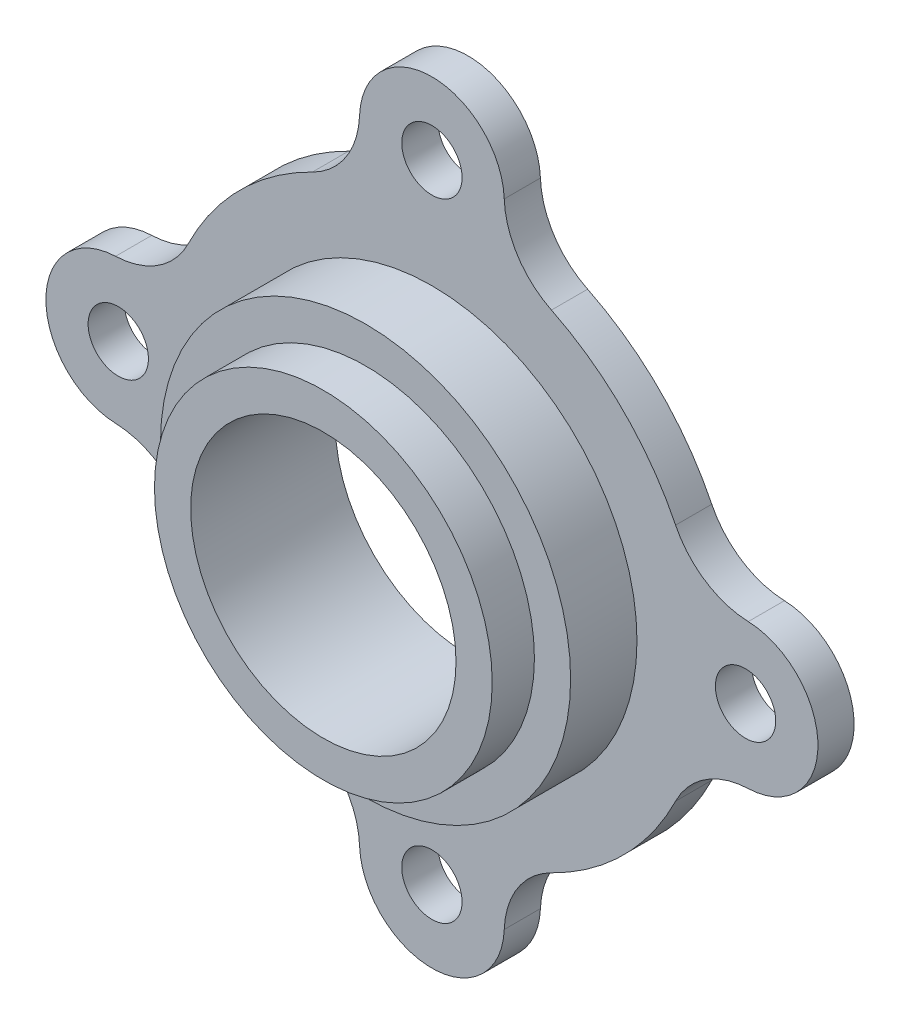
ISO-10303-21;
HEADER;
FILE_DESCRIPTION(('STEP AP214'),'2;1');
FILE_NAME('part.step','',(''),(''),'','','');
FILE_SCHEMA(('AUTOMOTIVE_DESIGN { 1 0 10303 214 1 1 1 1 }'));
ENDSEC;
DATA;
#1=APPLICATION_CONTEXT('core data for automotive mechanical design processes');
#2=APPLICATION_PROTOCOL_DEFINITION('international standard','automotive_design',2000,#1);
#3=PRODUCT_CONTEXT('',#1,'mechanical');
#4=PRODUCT('Part','Part','',(#3));
#5=PRODUCT_RELATED_PRODUCT_CATEGORY('part','',(#4));
#6=PRODUCT_DEFINITION_FORMATION('','',#4);
#7=PRODUCT_DEFINITION_CONTEXT('part definition',#1,'design');
#8=PRODUCT_DEFINITION('design','',#6,#7);
#9=PRODUCT_DEFINITION_SHAPE('','',#8);
#10=(LENGTH_UNIT() NAMED_UNIT(*) SI_UNIT(.MILLI.,.METRE.));
#11=(NAMED_UNIT(*) PLANE_ANGLE_UNIT() SI_UNIT($,.RADIAN.));
#12=(NAMED_UNIT(*) SI_UNIT($,.STERADIAN.) SOLID_ANGLE_UNIT());
#13=UNCERTAINTY_MEASURE_WITH_UNIT(LENGTH_MEASURE(1.E-05),#10,'distance_accuracy_value','');
#14=(GEOMETRIC_REPRESENTATION_CONTEXT(3) GLOBAL_UNCERTAINTY_ASSIGNED_CONTEXT((#13)) GLOBAL_UNIT_ASSIGNED_CONTEXT((#10,
#11,#12)) REPRESENTATION_CONTEXT('',''));
#15=CARTESIAN_POINT('',(0.,0.,0.));
#16=DIRECTION('',(0.,0.,1.));
#17=DIRECTION('',(1.,0.,0.));
#18=AXIS2_PLACEMENT_3D('',#15,#16,#17);
#19=CARTESIAN_POINT('',(12.9909281828426,26.4855769230769,3.));
#20=DIRECTION('',(0.,0.,-1.));
#21=DIRECTION('',(-1.,0.,0.));
#22=AXIS2_PLACEMENT_3D('',#19,#20,#21);
#23=CYLINDRICAL_SURFACE('',#22,7.);
#24=CARTESIAN_POINT('',(12.9909281828426,26.4855769230769,0.));
#25=DIRECTION('',(0.,0.,-1.));
#26=DIRECTION('',(-1.,0.,0.));
#27=AXIS2_PLACEMENT_3D('',#24,#25,#26);
#28=CIRCLE('',#27,7.);
#29=CARTESIAN_POINT('',(9.90833505471048,20.2008637548892,0.));
#30=VERTEX_POINT('',#29);
#31=CARTESIAN_POINT('',(5.99581300746583,26.2241124260355,0.));
#32=VERTEX_POINT('',#31);
#33=EDGE_CURVE('E186',#30,#32,#28,.T.);
#34=ORIENTED_EDGE('',*,*,#33,.T.);
#35=DIRECTION('',(0.,0.,-1.));
#36=VECTOR('',#35,1.);
#37=CARTESIAN_POINT('',(5.99581300746583,26.2241124260355,3.));
#38=LINE('',#37,#36);
#39=CARTESIAN_POINT('',(5.99581300746583,26.2241124260355,3.));
#40=VERTEX_POINT('',#39);
#41=EDGE_CURVE('E256',#40,#32,#38,.T.);
#42=ORIENTED_EDGE('',*,*,#41,.F.);
#43=CARTESIAN_POINT('',(12.9909281828426,26.4855769230769,3.));
#44=DIRECTION('',(0.,0.,-1.));
#45=DIRECTION('',(-1.,0.,0.));
#46=AXIS2_PLACEMENT_3D('',#43,#44,#45);
#47=CIRCLE('',#46,7.);
#48=CARTESIAN_POINT('',(9.90833505471048,20.2008637548892,3.));
#49=VERTEX_POINT('',#48);
#50=EDGE_CURVE('E222',#49,#40,#47,.T.);
#51=ORIENTED_EDGE('',*,*,#50,.F.);
#52=DIRECTION('',(0.,0.,-1.));
#53=VECTOR('',#52,1.);
#54=CARTESIAN_POINT('',(9.90833505471048,20.2008637548892,3.));
#55=LINE('',#54,#53);
#56=EDGE_CURVE('E188',#49,#30,#55,.T.);
#57=ORIENTED_EDGE('',*,*,#56,.T.);
#58=EDGE_LOOP('',(#34,#42,#51,#57));
#59=FACE_BOUND('',#58,.T.);
#60=ADVANCED_FACE('F43',(#59),#23,.F.);
#61=CARTESIAN_POINT('',(0.,26.,3.));
#62=DIRECTION('',(0.,0.,-1.));
#63=DIRECTION('',(-1.,0.,0.));
#64=AXIS2_PLACEMENT_3D('',#61,#62,#63);
#65=CYLINDRICAL_SURFACE('',#64,5.99999999999999);
#66=CARTESIAN_POINT('',(0.,26.,0.));
#67=DIRECTION('',(0.,0.,1.));
#68=DIRECTION('',(1.,0.,0.));
#69=AXIS2_PLACEMENT_3D('',#66,#67,#68);
#70=CIRCLE('',#69,5.99999999999999);
#71=CARTESIAN_POINT('',(-5.99581300746583,26.2241124260355,0.));
#72=VERTEX_POINT('',#71);
#73=EDGE_CURVE('E193',#32,#72,#70,.T.);
#74=ORIENTED_EDGE('',*,*,#73,.T.);
#75=DIRECTION('',(0.,0.,-1.));
#76=VECTOR('',#75,1.);
#77=CARTESIAN_POINT('',(-5.99581300746583,26.2241124260355,3.));
#78=LINE('',#77,#76);
#79=CARTESIAN_POINT('',(-5.99581300746583,26.2241124260355,3.));
#80=VERTEX_POINT('',#79);
#81=EDGE_CURVE('E254',#80,#72,#78,.T.);
#82=ORIENTED_EDGE('',*,*,#81,.F.);
#83=CARTESIAN_POINT('',(0.,26.,3.));
#84=DIRECTION('',(0.,0.,1.));
#85=DIRECTION('',(1.,0.,0.));
#86=AXIS2_PLACEMENT_3D('',#83,#84,#85);
#87=CIRCLE('',#86,5.99999999999999);
#88=EDGE_CURVE('E129',#40,#80,#87,.T.);
#89=ORIENTED_EDGE('',*,*,#88,.F.);
#90=ORIENTED_EDGE('',*,*,#41,.T.);
#91=EDGE_LOOP('',(#74,#82,#89,#90));
#92=FACE_BOUND('',#91,.T.);
#93=ADVANCED_FACE('F345',(#92),#65,.T.);
#94=CARTESIAN_POINT('',(-12.9909281828426,26.4855769230769,3.));
#95=DIRECTION('',(0.,0.,-1.));
#96=DIRECTION('',(-1.,0.,0.));
#97=AXIS2_PLACEMENT_3D('',#94,#95,#96);
#98=CYLINDRICAL_SURFACE('',#97,7.);
#99=CARTESIAN_POINT('',(-12.9909281828426,26.4855769230769,0.));
#100=DIRECTION('',(0.,0.,-1.));
#101=DIRECTION('',(-1.,0.,0.));
#102=AXIS2_PLACEMENT_3D('',#99,#100,#101);
#103=CIRCLE('',#102,7.);
#104=CARTESIAN_POINT('',(-9.90833505471049,20.2008637548892,0.));
#105=VERTEX_POINT('',#104);
#106=EDGE_CURVE('E198',#72,#105,#103,.T.);
#107=ORIENTED_EDGE('',*,*,#106,.T.);
#108=DIRECTION('',(0.,0.,-1.));
#109=VECTOR('',#108,1.);
#110=CARTESIAN_POINT('',(-9.90833505471049,20.2008637548892,3.));
#111=LINE('',#110,#109);
#112=CARTESIAN_POINT('',(-9.90833505471049,20.2008637548892,3.));
#113=VERTEX_POINT('',#112);
#114=EDGE_CURVE('E252',#113,#105,#111,.T.);
#115=ORIENTED_EDGE('',*,*,#114,.F.);
#116=CARTESIAN_POINT('',(-12.9909281828426,26.4855769230769,3.));
#117=DIRECTION('',(0.,0.,-1.));
#118=DIRECTION('',(-1.,0.,0.));
#119=AXIS2_PLACEMENT_3D('',#116,#117,#118);
#120=CIRCLE('',#119,7.);
#121=EDGE_CURVE('E294',#80,#113,#120,.T.);
#122=ORIENTED_EDGE('',*,*,#121,.F.);
#123=ORIENTED_EDGE('',*,*,#81,.T.);
#124=EDGE_LOOP('',(#107,#115,#122,#123));
#125=FACE_BOUND('',#124,.T.);
#126=ADVANCED_FACE('F347',(#125),#98,.F.);
#127=CARTESIAN_POINT('',(0.,0.,3.));
#128=DIRECTION('',(0.,0.,-1.));
#129=DIRECTION('',(-1.,0.,0.));
#130=AXIS2_PLACEMENT_3D('',#127,#128,#129);
#131=CYLINDRICAL_SURFACE('',#130,22.5);
#132=CARTESIAN_POINT('',(0.,0.,0.));
#133=DIRECTION('',(0.,0.,1.));
#134=DIRECTION('',(1.,0.,0.));
#135=AXIS2_PLACEMENT_3D('',#132,#133,#134);
#136=CIRCLE('',#135,22.5);
#137=CARTESIAN_POINT('',(-20.2008637548892,9.90833505471048,0.));
#138=VERTEX_POINT('',#137);
#139=EDGE_CURVE('E196',#105,#138,#136,.T.);
#140=ORIENTED_EDGE('',*,*,#139,.T.);
#141=DIRECTION('',(0.,0.,-1.));
#142=VECTOR('',#141,1.);
#143=CARTESIAN_POINT('',(-20.2008637548892,9.90833505471048,3.));
#144=LINE('',#143,#142);
#145=CARTESIAN_POINT('',(-20.2008637548892,9.90833505471048,3.));
#146=VERTEX_POINT('',#145);
#147=EDGE_CURVE('E249',#146,#138,#144,.T.);
#148=ORIENTED_EDGE('',*,*,#147,.F.);
#149=CARTESIAN_POINT('',(0.,0.,3.));
#150=DIRECTION('',(0.,0.,1.));
#151=DIRECTION('',(1.,0.,0.));
#152=AXIS2_PLACEMENT_3D('',#149,#150,#151);
#153=CIRCLE('',#152,22.5);
#154=EDGE_CURVE('E298',#113,#146,#153,.T.);
#155=ORIENTED_EDGE('',*,*,#154,.F.);
#156=ORIENTED_EDGE('',*,*,#114,.T.);
#157=EDGE_LOOP('',(#140,#148,#155,#156));
#158=FACE_BOUND('',#157,.T.);
#159=ADVANCED_FACE('F348',(#158),#131,.T.);
#160=CARTESIAN_POINT('',(-26.4855769230769,12.9909281828426,3.));
#161=DIRECTION('',(0.,0.,-1.));
#162=DIRECTION('',(-1.,0.,0.));
#163=AXIS2_PLACEMENT_3D('',#160,#161,#162);
#164=CYLINDRICAL_SURFACE('',#163,7.);
#165=CARTESIAN_POINT('',(-26.4855769230769,12.9909281828426,0.));
#166=DIRECTION('',(0.,0.,-1.));
#167=DIRECTION('',(-1.,0.,0.));
#168=AXIS2_PLACEMENT_3D('',#165,#166,#167);
#169=CIRCLE('',#168,7.);
#170=CARTESIAN_POINT('',(-26.2241124260355,5.99581300746583,0.));
#171=VERTEX_POINT('',#170);
#172=EDGE_CURVE('E199',#138,#171,#169,.T.);
#173=ORIENTED_EDGE('',*,*,#172,.T.);
#174=DIRECTION('',(0.,0.,-1.));
#175=VECTOR('',#174,1.);
#176=CARTESIAN_POINT('',(-26.2241124260355,5.99581300746583,3.));
#177=LINE('',#176,#175);
#178=CARTESIAN_POINT('',(-26.2241124260355,5.99581300746583,3.));
#179=VERTEX_POINT('',#178);
#180=EDGE_CURVE('E247',#179,#171,#177,.T.);
#181=ORIENTED_EDGE('',*,*,#180,.F.);
#182=CARTESIAN_POINT('',(-26.4855769230769,12.9909281828426,3.));
#183=DIRECTION('',(0.,0.,-1.));
#184=DIRECTION('',(-1.,0.,0.));
#185=AXIS2_PLACEMENT_3D('',#182,#183,#184);
#186=CIRCLE('',#185,7.);
#187=EDGE_CURVE('E297',#146,#179,#186,.T.);
#188=ORIENTED_EDGE('',*,*,#187,.F.);
#189=ORIENTED_EDGE('',*,*,#147,.T.);
#190=EDGE_LOOP('',(#173,#181,#188,#189));
#191=FACE_BOUND('',#190,.T.);
#192=ADVANCED_FACE('F357',(#191),#164,.F.);
#193=CARTESIAN_POINT('',(-26.,0.,3.));
#194=DIRECTION('',(0.,0.,-1.));
#195=DIRECTION('',(-1.,0.,0.));
#196=AXIS2_PLACEMENT_3D('',#193,#194,#195);
#197=CYLINDRICAL_SURFACE('',#196,5.99999999999999);
#198=CARTESIAN_POINT('',(-26.,0.,0.));
#199=DIRECTION('',(0.,0.,1.));
#200=DIRECTION('',(1.,0.,0.));
#201=AXIS2_PLACEMENT_3D('',#198,#199,#200);
#202=CIRCLE('',#201,5.99999999999999);
#203=CARTESIAN_POINT('',(-26.2241124260355,-5.99581300746583,0.));
#204=VERTEX_POINT('',#203);
#205=EDGE_CURVE('E205',#171,#204,#202,.T.);
#206=ORIENTED_EDGE('',*,*,#205,.T.);
#207=DIRECTION('',(0.,0.,-1.));
#208=VECTOR('',#207,1.);
#209=CARTESIAN_POINT('',(-26.2241124260355,-5.99581300746583,3.));
#210=LINE('',#209,#208);
#211=CARTESIAN_POINT('',(-26.2241124260355,-5.99581300746583,3.));
#212=VERTEX_POINT('',#211);
#213=EDGE_CURVE('E242',#212,#204,#210,.T.);
#214=ORIENTED_EDGE('',*,*,#213,.F.);
#215=CARTESIAN_POINT('',(-26.,0.,3.));
#216=DIRECTION('',(0.,0.,1.));
#217=DIRECTION('',(1.,0.,0.));
#218=AXIS2_PLACEMENT_3D('',#215,#216,#217);
#219=CIRCLE('',#218,5.99999999999999);
#220=EDGE_CURVE('E296',#179,#212,#219,.T.);
#221=ORIENTED_EDGE('',*,*,#220,.F.);
#222=ORIENTED_EDGE('',*,*,#180,.T.);
#223=EDGE_LOOP('',(#206,#214,#221,#222));
#224=FACE_BOUND('',#223,.T.);
#225=ADVANCED_FACE('F356',(#224),#197,.T.);
#226=CARTESIAN_POINT('',(-26.4855769230769,-12.9909281828426,3.));
#227=DIRECTION('',(0.,0.,-1.));
#228=DIRECTION('',(-1.,0.,0.));
#229=AXIS2_PLACEMENT_3D('',#226,#227,#228);
#230=CYLINDRICAL_SURFACE('',#229,7.);
#231=CARTESIAN_POINT('',(-26.4855769230769,-12.9909281828426,0.));
#232=DIRECTION('',(0.,0.,-1.));
#233=DIRECTION('',(1.,0.,0.));
#234=AXIS2_PLACEMENT_3D('',#231,#232,#233);
#235=CIRCLE('',#234,7.);
#236=CARTESIAN_POINT('',(-20.2008637548892,-9.90833505471048,0.));
#237=VERTEX_POINT('',#236);
#238=EDGE_CURVE('E204',#204,#237,#235,.T.);
#239=ORIENTED_EDGE('',*,*,#238,.T.);
#240=DIRECTION('',(0.,0.,-1.));
#241=VECTOR('',#240,1.);
#242=CARTESIAN_POINT('',(-20.2008637548892,-9.90833505471048,3.));
#243=LINE('',#242,#241);
#244=CARTESIAN_POINT('',(-20.2008637548892,-9.90833505471048,3.));
#245=VERTEX_POINT('',#244);
#246=EDGE_CURVE('E238',#245,#237,#243,.T.);
#247=ORIENTED_EDGE('',*,*,#246,.F.);
#248=CARTESIAN_POINT('',(-26.4855769230769,-12.9909281828426,3.));
#249=DIRECTION('',(0.,0.,-1.));
#250=DIRECTION('',(1.,0.,0.));
#251=AXIS2_PLACEMENT_3D('',#248,#249,#250);
#252=CIRCLE('',#251,7.);
#253=EDGE_CURVE('E305',#212,#245,#252,.T.);
#254=ORIENTED_EDGE('',*,*,#253,.F.);
#255=ORIENTED_EDGE('',*,*,#213,.T.);
#256=EDGE_LOOP('',(#239,#247,#254,#255));
#257=FACE_BOUND('',#256,.T.);
#258=ADVANCED_FACE('F365',(#257),#230,.F.);
#259=CARTESIAN_POINT('',(0.,0.,3.));
#260=DIRECTION('',(0.,0.,-1.));
#261=DIRECTION('',(-1.,0.,0.));
#262=AXIS2_PLACEMENT_3D('',#259,#260,#261);
#263=CYLINDRICAL_SURFACE('',#262,22.5);
#264=CARTESIAN_POINT('',(0.,0.,0.));
#265=DIRECTION('',(0.,0.,1.));
#266=DIRECTION('',(1.,0.,0.));
#267=AXIS2_PLACEMENT_3D('',#264,#265,#266);
#268=CIRCLE('',#267,22.5);
#269=CARTESIAN_POINT('',(-9.90833505471048,-20.2008637548892,0.));
#270=VERTEX_POINT('',#269);
#271=EDGE_CURVE('E206',#237,#270,#268,.T.);
#272=ORIENTED_EDGE('',*,*,#271,.T.);
#273=DIRECTION('',(0.,0.,-1.));
#274=VECTOR('',#273,1.);
#275=CARTESIAN_POINT('',(-9.90833505471048,-20.2008637548892,3.));
#276=LINE('',#275,#274);
#277=CARTESIAN_POINT('',(-9.90833505471048,-20.2008637548892,3.));
#278=VERTEX_POINT('',#277);
#279=EDGE_CURVE('E240',#278,#270,#276,.T.);
#280=ORIENTED_EDGE('',*,*,#279,.F.);
#281=CARTESIAN_POINT('',(0.,0.,3.));
#282=DIRECTION('',(0.,0.,1.));
#283=DIRECTION('',(1.,0.,0.));
#284=AXIS2_PLACEMENT_3D('',#281,#282,#283);
#285=CIRCLE('',#284,22.5);
#286=EDGE_CURVE('E304',#245,#278,#285,.T.);
#287=ORIENTED_EDGE('',*,*,#286,.F.);
#288=ORIENTED_EDGE('',*,*,#246,.T.);
#289=EDGE_LOOP('',(#272,#280,#287,#288));
#290=FACE_BOUND('',#289,.T.);
#291=ADVANCED_FACE('F366',(#290),#263,.T.);
#292=CARTESIAN_POINT('',(-12.9909281828426,-26.4855769230769,3.));
#293=DIRECTION('',(0.,0.,-1.));
#294=DIRECTION('',(-1.,0.,0.));
#295=AXIS2_PLACEMENT_3D('',#292,#293,#294);
#296=CYLINDRICAL_SURFACE('',#295,7.);
#297=CARTESIAN_POINT('',(-12.9909281828426,-26.4855769230769,0.));
#298=DIRECTION('',(0.,0.,-1.));
#299=DIRECTION('',(1.,0.,0.));
#300=AXIS2_PLACEMENT_3D('',#297,#298,#299);
#301=CIRCLE('',#300,7.);
#302=CARTESIAN_POINT('',(-5.99581300746583,-26.2241124260355,0.));
#303=VERTEX_POINT('',#302);
#304=EDGE_CURVE('E208',#270,#303,#301,.T.);
#305=ORIENTED_EDGE('',*,*,#304,.T.);
#306=DIRECTION('',(0.,0.,-1.));
#307=VECTOR('',#306,1.);
#308=CARTESIAN_POINT('',(-5.99581300746583,-26.2241124260355,3.));
#309=LINE('',#308,#307);
#310=CARTESIAN_POINT('',(-5.99581300746583,-26.2241124260355,3.));
#311=VERTEX_POINT('',#310);
#312=EDGE_CURVE('E234',#311,#303,#309,.T.);
#313=ORIENTED_EDGE('',*,*,#312,.F.);
#314=CARTESIAN_POINT('',(-12.9909281828426,-26.4855769230769,3.));
#315=DIRECTION('',(0.,0.,-1.));
#316=DIRECTION('',(1.,0.,0.));
#317=AXIS2_PLACEMENT_3D('',#314,#315,#316);
#318=CIRCLE('',#317,7.);
#319=EDGE_CURVE('E308',#278,#311,#318,.T.);
#320=ORIENTED_EDGE('',*,*,#319,.F.);
#321=ORIENTED_EDGE('',*,*,#279,.T.);
#322=EDGE_LOOP('',(#305,#313,#320,#321));
#323=FACE_BOUND('',#322,.T.);
#324=ADVANCED_FACE('F375',(#323),#296,.F.);
#325=CARTESIAN_POINT('',(0.,-26.,3.));
#326=DIRECTION('',(0.,0.,-1.));
#327=DIRECTION('',(-1.,0.,0.));
#328=AXIS2_PLACEMENT_3D('',#325,#326,#327);
#329=CYLINDRICAL_SURFACE('',#328,5.99999999999999);
#330=CARTESIAN_POINT('',(0.,-26.,0.));
#331=DIRECTION('',(0.,0.,1.));
#332=DIRECTION('',(1.,0.,0.));
#333=AXIS2_PLACEMENT_3D('',#330,#331,#332);
#334=CIRCLE('',#333,5.99999999999999);
#335=CARTESIAN_POINT('',(5.99581300746583,-26.2241124260355,0.));
#336=VERTEX_POINT('',#335);
#337=EDGE_CURVE('E209',#303,#336,#334,.T.);
#338=ORIENTED_EDGE('',*,*,#337,.T.);
#339=DIRECTION('',(0.,0.,-1.));
#340=VECTOR('',#339,1.);
#341=CARTESIAN_POINT('',(5.99581300746583,-26.2241124260355,3.));
#342=LINE('',#341,#340);
#343=CARTESIAN_POINT('',(5.99581300746583,-26.2241124260355,3.));
#344=VERTEX_POINT('',#343);
#345=EDGE_CURVE('E232',#344,#336,#342,.T.);
#346=ORIENTED_EDGE('',*,*,#345,.F.);
#347=CARTESIAN_POINT('',(0.,-26.,3.));
#348=DIRECTION('',(0.,0.,1.));
#349=DIRECTION('',(1.,0.,0.));
#350=AXIS2_PLACEMENT_3D('',#347,#348,#349);
#351=CIRCLE('',#350,5.99999999999999);
#352=EDGE_CURVE('E306',#311,#344,#351,.T.);
#353=ORIENTED_EDGE('',*,*,#352,.F.);
#354=ORIENTED_EDGE('',*,*,#312,.T.);
#355=EDGE_LOOP('',(#338,#346,#353,#354));
#356=FACE_BOUND('',#355,.T.);
#357=ADVANCED_FACE('F376',(#356),#329,.T.);
#358=CARTESIAN_POINT('',(12.9909281828426,-26.4855769230769,3.));
#359=DIRECTION('',(0.,0.,-1.));
#360=DIRECTION('',(-1.,0.,0.));
#361=AXIS2_PLACEMENT_3D('',#358,#359,#360);
#362=CYLINDRICAL_SURFACE('',#361,7.);
#363=CARTESIAN_POINT('',(12.9909281828426,-26.4855769230769,0.));
#364=DIRECTION('',(0.,0.,-1.));
#365=DIRECTION('',(1.,0.,0.));
#366=AXIS2_PLACEMENT_3D('',#363,#364,#365);
#367=CIRCLE('',#366,7.);
#368=CARTESIAN_POINT('',(9.90833505471048,-20.2008637548892,0.));
#369=VERTEX_POINT('',#368);
#370=EDGE_CURVE('E215',#336,#369,#367,.T.);
#371=ORIENTED_EDGE('',*,*,#370,.T.);
#372=DIRECTION('',(0.,0.,-1.));
#373=VECTOR('',#372,1.);
#374=CARTESIAN_POINT('',(9.90833505471048,-20.2008637548892,3.));
#375=LINE('',#374,#373);
#376=CARTESIAN_POINT('',(9.90833505471048,-20.2008637548892,3.));
#377=VERTEX_POINT('',#376);
#378=EDGE_CURVE('E227',#377,#369,#375,.T.);
#379=ORIENTED_EDGE('',*,*,#378,.F.);
#380=CARTESIAN_POINT('',(12.9909281828426,-26.4855769230769,3.));
#381=DIRECTION('',(0.,0.,-1.));
#382=DIRECTION('',(1.,0.,0.));
#383=AXIS2_PLACEMENT_3D('',#380,#381,#382);
#384=CIRCLE('',#383,7.);
#385=EDGE_CURVE('E309',#344,#377,#384,.T.);
#386=ORIENTED_EDGE('',*,*,#385,.F.);
#387=ORIENTED_EDGE('',*,*,#345,.T.);
#388=EDGE_LOOP('',(#371,#379,#386,#387));
#389=FACE_BOUND('',#388,.T.);
#390=ADVANCED_FACE('F379',(#389),#362,.F.);
#391=CARTESIAN_POINT('',(0.,0.,3.));
#392=DIRECTION('',(0.,0.,-1.));
#393=DIRECTION('',(-1.,0.,0.));
#394=AXIS2_PLACEMENT_3D('',#391,#392,#393);
#395=CYLINDRICAL_SURFACE('',#394,22.5);
#396=CARTESIAN_POINT('',(0.,0.,0.));
#397=DIRECTION('',(0.,0.,1.));
#398=DIRECTION('',(1.,0.,0.));
#399=AXIS2_PLACEMENT_3D('',#396,#397,#398);
#400=CIRCLE('',#399,22.5);
#401=CARTESIAN_POINT('',(20.2008637548892,-9.90833505471048,0.));
#402=VERTEX_POINT('',#401);
#403=EDGE_CURVE('E212',#369,#402,#400,.T.);
#404=ORIENTED_EDGE('',*,*,#403,.T.);
#405=DIRECTION('',(0.,0.,-1.));
#406=VECTOR('',#405,1.);
#407=CARTESIAN_POINT('',(20.2008637548892,-9.90833505471048,3.));
#408=LINE('',#407,#406);
#409=CARTESIAN_POINT('',(20.2008637548892,-9.90833505471048,3.));
#410=VERTEX_POINT('',#409);
#411=EDGE_CURVE('E223',#410,#402,#408,.T.);
#412=ORIENTED_EDGE('',*,*,#411,.F.);
#413=CARTESIAN_POINT('',(0.,0.,3.));
#414=DIRECTION('',(0.,0.,1.));
#415=DIRECTION('',(1.,0.,0.));
#416=AXIS2_PLACEMENT_3D('',#413,#414,#415);
#417=CIRCLE('',#416,22.5);
#418=EDGE_CURVE('E315',#377,#410,#417,.T.);
#419=ORIENTED_EDGE('',*,*,#418,.F.);
#420=ORIENTED_EDGE('',*,*,#378,.T.);
#421=EDGE_LOOP('',(#404,#412,#419,#420));
#422=FACE_BOUND('',#421,.T.);
#423=ADVANCED_FACE('F318',(#422),#395,.T.);
#424=CARTESIAN_POINT('',(26.4855769230769,-12.9909281828426,3.));
#425=DIRECTION('',(0.,0.,-1.));
#426=DIRECTION('',(-1.,0.,0.));
#427=AXIS2_PLACEMENT_3D('',#424,#425,#426);
#428=CYLINDRICAL_SURFACE('',#427,7.);
#429=CARTESIAN_POINT('',(26.4855769230769,-12.9909281828426,0.));
#430=DIRECTION('',(0.,0.,-1.));
#431=DIRECTION('',(1.,0.,0.));
#432=AXIS2_PLACEMENT_3D('',#429,#430,#431);
#433=CIRCLE('',#432,7.);
#434=CARTESIAN_POINT('',(26.2241124260355,-5.99581300746583,0.));
#435=VERTEX_POINT('',#434);
#436=EDGE_CURVE('E216',#402,#435,#433,.T.);
#437=ORIENTED_EDGE('',*,*,#436,.T.);
#438=DIRECTION('',(0.,0.,-1.));
#439=VECTOR('',#438,1.);
#440=CARTESIAN_POINT('',(26.2241124260355,-5.99581300746583,3.));
#441=LINE('',#440,#439);
#442=CARTESIAN_POINT('',(26.2241124260355,-5.99581300746583,3.));
#443=VERTEX_POINT('',#442);
#444=EDGE_CURVE('E182',#443,#435,#441,.T.);
#445=ORIENTED_EDGE('',*,*,#444,.F.);
#446=CARTESIAN_POINT('',(26.4855769230769,-12.9909281828426,3.));
#447=DIRECTION('',(0.,0.,-1.));
#448=DIRECTION('',(1.,0.,0.));
#449=AXIS2_PLACEMENT_3D('',#446,#447,#448);
#450=CIRCLE('',#449,7.);
#451=EDGE_CURVE('E174',#410,#443,#450,.T.);
#452=ORIENTED_EDGE('',*,*,#451,.F.);
#453=ORIENTED_EDGE('',*,*,#411,.T.);
#454=EDGE_LOOP('',(#437,#445,#452,#453));
#455=FACE_BOUND('',#454,.T.);
#456=ADVANCED_FACE('F325',(#455),#428,.F.);
#457=CARTESIAN_POINT('',(26.,0.,3.));
#458=DIRECTION('',(0.,0.,-1.));
#459=DIRECTION('',(-1.,0.,0.));
#460=AXIS2_PLACEMENT_3D('',#457,#458,#459);
#461=CYLINDRICAL_SURFACE('',#460,5.99999999999999);
#462=CARTESIAN_POINT('',(26.,0.,0.));
#463=DIRECTION('',(0.,0.,1.));
#464=DIRECTION('',(1.,0.,0.));
#465=AXIS2_PLACEMENT_3D('',#462,#463,#464);
#466=CIRCLE('',#465,5.99999999999999);
#467=CARTESIAN_POINT('',(26.2241124260355,5.99581300746583,0.));
#468=VERTEX_POINT('',#467);
#469=EDGE_CURVE('E176',#435,#468,#466,.T.);
#470=ORIENTED_EDGE('',*,*,#469,.T.);
#471=DIRECTION('',(0.,0.,-1.));
#472=VECTOR('',#471,1.);
#473=CARTESIAN_POINT('',(26.2241124260355,5.99581300746583,3.));
#474=LINE('',#473,#472);
#475=CARTESIAN_POINT('',(26.2241124260355,5.99581300746583,3.));
#476=VERTEX_POINT('',#475);
#477=EDGE_CURVE('E180',#476,#468,#474,.T.);
#478=ORIENTED_EDGE('',*,*,#477,.F.);
#479=CARTESIAN_POINT('',(26.,0.,3.));
#480=DIRECTION('',(0.,0.,1.));
#481=DIRECTION('',(1.,0.,0.));
#482=AXIS2_PLACEMENT_3D('',#479,#480,#481);
#483=CIRCLE('',#482,5.99999999999999);
#484=EDGE_CURVE('E167',#443,#476,#483,.T.);
#485=ORIENTED_EDGE('',*,*,#484,.F.);
#486=ORIENTED_EDGE('',*,*,#444,.T.);
#487=EDGE_LOOP('',(#470,#478,#485,#486));
#488=FACE_BOUND('',#487,.T.);
#489=ADVANCED_FACE('F178',(#488),#461,.T.);
#490=CARTESIAN_POINT('',(26.4855769230769,12.9909281828426,3.));
#491=DIRECTION('',(0.,0.,-1.));
#492=DIRECTION('',(-1.,0.,0.));
#493=AXIS2_PLACEMENT_3D('',#490,#491,#492);
#494=CYLINDRICAL_SURFACE('',#493,7.);
#495=CARTESIAN_POINT('',(26.4855769230769,12.9909281828426,0.));
#496=DIRECTION('',(0.,0.,-1.));
#497=DIRECTION('',(-1.,0.,0.));
#498=AXIS2_PLACEMENT_3D('',#495,#496,#497);
#499=CIRCLE('',#498,7.);
#500=CARTESIAN_POINT('',(20.2008637548892,9.90833505471048,0.));
#501=VERTEX_POINT('',#500);
#502=EDGE_CURVE('E111',#468,#501,#499,.T.);
#503=ORIENTED_EDGE('',*,*,#502,.T.);
#504=DIRECTION('',(0.,0.,-1.));
#505=VECTOR('',#504,1.);
#506=CARTESIAN_POINT('',(20.2008637548892,9.90833505471048,3.));
#507=LINE('',#506,#505);
#508=CARTESIAN_POINT('',(20.2008637548892,9.90833505471048,3.));
#509=VERTEX_POINT('',#508);
#510=EDGE_CURVE('E185',#509,#501,#507,.T.);
#511=ORIENTED_EDGE('',*,*,#510,.F.);
#512=CARTESIAN_POINT('',(26.4855769230769,12.9909281828426,3.));
#513=DIRECTION('',(0.,0.,-1.));
#514=DIRECTION('',(-1.,0.,0.));
#515=AXIS2_PLACEMENT_3D('',#512,#513,#514);
#516=CIRCLE('',#515,7.);
#517=EDGE_CURVE('E168',#476,#509,#516,.T.);
#518=ORIENTED_EDGE('',*,*,#517,.F.);
#519=ORIENTED_EDGE('',*,*,#477,.T.);
#520=EDGE_LOOP('',(#503,#511,#518,#519));
#521=FACE_BOUND('',#520,.T.);
#522=ADVANCED_FACE('F184',(#521),#494,.F.);
#523=CARTESIAN_POINT('',(0.,0.,3.));
#524=DIRECTION('',(0.,0.,-1.));
#525=DIRECTION('',(-1.,0.,0.));
#526=AXIS2_PLACEMENT_3D('',#523,#524,#525);
#527=CYLINDRICAL_SURFACE('',#526,22.5);
#528=CARTESIAN_POINT('',(0.,0.,0.));
#529=DIRECTION('',(0.,0.,1.));
#530=DIRECTION('',(1.,0.,0.));
#531=AXIS2_PLACEMENT_3D('',#528,#529,#530);
#532=CIRCLE('',#531,22.5);
#533=EDGE_CURVE('E116',#501,#30,#532,.T.);
#534=ORIENTED_EDGE('',*,*,#533,.T.);
#535=ORIENTED_EDGE('',*,*,#56,.F.);
#536=CARTESIAN_POINT('',(0.,0.,3.));
#537=DIRECTION('',(0.,0.,1.));
#538=DIRECTION('',(1.,0.,0.));
#539=AXIS2_PLACEMENT_3D('',#536,#537,#538);
#540=CIRCLE('',#539,22.5);
#541=EDGE_CURVE('E63',#509,#49,#540,.T.);
#542=ORIENTED_EDGE('',*,*,#541,.F.);
#543=ORIENTED_EDGE('',*,*,#510,.T.);
#544=EDGE_LOOP('',(#534,#535,#542,#543));
#545=FACE_BOUND('',#544,.T.);
#546=ADVANCED_FACE('F329',(#545),#527,.T.);
#547=CARTESIAN_POINT('',(6.49546409142132,26.2427884615385,3.));
#548=DIRECTION('',(0.,0.,-1.));
#549=DIRECTION('',(-1.,0.,0.));
#550=AXIS2_PLACEMENT_3D('',#547,#548,#549);
#551=PLANE('',#550);
#552=CARTESIAN_POINT('',(-26.,0.,3.));
#553=DIRECTION('',(0.,0.,1.));
#554=DIRECTION('',(1.,0.,0.));
#555=AXIS2_PLACEMENT_3D('',#552,#553,#554);
#556=CIRCLE('',#555,2.5);
#557=CARTESIAN_POINT('',(-23.5,0.,3.));
#558=VERTEX_POINT('',#557);
#559=EDGE_CURVE('E266',#558,#558,#556,.T.);
#560=ORIENTED_EDGE('',*,*,#559,.F.);
#561=EDGE_LOOP('',(#560));
#562=FACE_BOUND('',#561,.T.);
#563=CARTESIAN_POINT('',(0.,26.,3.));
#564=DIRECTION('',(0.,0.,1.));
#565=DIRECTION('',(1.,0.,0.));
#566=AXIS2_PLACEMENT_3D('',#563,#564,#565);
#567=CIRCLE('',#566,2.5);
#568=CARTESIAN_POINT('',(2.5,26.,3.));
#569=VERTEX_POINT('',#568);
#570=EDGE_CURVE('E691',#569,#569,#567,.T.);
#571=ORIENTED_EDGE('',*,*,#570,.F.);
#572=EDGE_LOOP('',(#571));
#573=FACE_BOUND('',#572,.T.);
#574=CARTESIAN_POINT('',(26.,0.,3.));
#575=DIRECTION('',(0.,0.,1.));
#576=DIRECTION('',(1.,0.,0.));
#577=AXIS2_PLACEMENT_3D('',#574,#575,#576);
#578=CIRCLE('',#577,2.5);
#579=CARTESIAN_POINT('',(28.5,0.,3.));
#580=VERTEX_POINT('',#579);
#581=EDGE_CURVE('E698',#580,#580,#578,.T.);
#582=ORIENTED_EDGE('',*,*,#581,.F.);
#583=EDGE_LOOP('',(#582));
#584=FACE_BOUND('',#583,.T.);
#585=CARTESIAN_POINT('',(0.,-26.,3.));
#586=DIRECTION('',(0.,0.,1.));
#587=DIRECTION('',(1.,0.,0.));
#588=AXIS2_PLACEMENT_3D('',#585,#586,#587);
#589=CIRCLE('',#588,2.5);
#590=CARTESIAN_POINT('',(2.5,-26.,3.));
#591=VERTEX_POINT('',#590);
#592=EDGE_CURVE('E281',#591,#591,#589,.T.);
#593=ORIENTED_EDGE('',*,*,#592,.F.);
#594=EDGE_LOOP('',(#593));
#595=FACE_BOUND('',#594,.T.);
#596=CARTESIAN_POINT('',(0.,0.,3.));
#597=DIRECTION('',(0.,0.,-1.));
#598=DIRECTION('',(-1.,0.,0.));
#599=AXIS2_PLACEMENT_3D('',#596,#597,#598);
#600=CIRCLE('',#599,17.);
#601=CARTESIAN_POINT('',(-17.,0.,3.));
#602=VERTEX_POINT('',#601);
#603=EDGE_CURVE('E55',#602,#602,#600,.F.);
#604=ORIENTED_EDGE('',*,*,#603,.F.);
#605=EDGE_LOOP('',(#604));
#606=FACE_BOUND('',#605,.T.);
#607=ORIENTED_EDGE('',*,*,#50,.T.);
#608=ORIENTED_EDGE('',*,*,#88,.T.);
#609=ORIENTED_EDGE('',*,*,#121,.T.);
#610=ORIENTED_EDGE('',*,*,#154,.T.);
#611=ORIENTED_EDGE('',*,*,#187,.T.);
#612=ORIENTED_EDGE('',*,*,#220,.T.);
#613=ORIENTED_EDGE('',*,*,#253,.T.);
#614=ORIENTED_EDGE('',*,*,#286,.T.);
#615=ORIENTED_EDGE('',*,*,#319,.T.);
#616=ORIENTED_EDGE('',*,*,#352,.T.);
#617=ORIENTED_EDGE('',*,*,#385,.T.);
#618=ORIENTED_EDGE('',*,*,#418,.T.);
#619=ORIENTED_EDGE('',*,*,#451,.T.);
#620=ORIENTED_EDGE('',*,*,#484,.T.);
#621=ORIENTED_EDGE('',*,*,#517,.T.);
#622=ORIENTED_EDGE('',*,*,#541,.T.);
#623=EDGE_LOOP('',(#607,#608,#609,#610,#611,#612,#613,#614,#615,#616,#617,#618,#619,#620,#621,#622));
#624=FACE_BOUND('',#623,.T.);
#625=ADVANCED_FACE('F169',(#562,#573,#584,#595,#606,#624),#551,.F.);
#626=CARTESIAN_POINT('',(6.49546409142132,26.2427884615385,0.));
#627=DIRECTION('',(0.,0.,-1.));
#628=DIRECTION('',(-1.,0.,0.));
#629=AXIS2_PLACEMENT_3D('',#626,#627,#628);
#630=PLANE('',#629);
#631=CARTESIAN_POINT('',(-26.,0.,0.));
#632=DIRECTION('',(0.,0.,-1.));
#633=DIRECTION('',(-1.,0.,0.));
#634=AXIS2_PLACEMENT_3D('',#631,#632,#633);
#635=CIRCLE('',#634,2.5);
#636=CARTESIAN_POINT('',(-28.5,0.,0.));
#637=VERTEX_POINT('',#636);
#638=EDGE_CURVE('E46',#637,#637,#635,.T.);
#639=ORIENTED_EDGE('',*,*,#638,.F.);
#640=EDGE_LOOP('',(#639));
#641=FACE_BOUND('',#640,.T.);
#642=CARTESIAN_POINT('',(0.,26.,0.));
#643=DIRECTION('',(0.,0.,-1.));
#644=DIRECTION('',(-1.,0.,0.));
#645=AXIS2_PLACEMENT_3D('',#642,#643,#644);
#646=CIRCLE('',#645,2.5);
#647=CARTESIAN_POINT('',(-2.5,26.,0.));
#648=VERTEX_POINT('',#647);
#649=EDGE_CURVE('E268',#648,#648,#646,.T.);
#650=ORIENTED_EDGE('',*,*,#649,.F.);
#651=EDGE_LOOP('',(#650));
#652=FACE_BOUND('',#651,.T.);
#653=CARTESIAN_POINT('',(26.,0.,0.));
#654=DIRECTION('',(0.,0.,-1.));
#655=DIRECTION('',(-1.,0.,0.));
#656=AXIS2_PLACEMENT_3D('',#653,#654,#655);
#657=CIRCLE('',#656,2.5);
#658=CARTESIAN_POINT('',(23.5,0.,0.));
#659=VERTEX_POINT('',#658);
#660=EDGE_CURVE('E264',#659,#659,#657,.T.);
#661=ORIENTED_EDGE('',*,*,#660,.F.);
#662=EDGE_LOOP('',(#661));
#663=FACE_BOUND('',#662,.T.);
#664=CARTESIAN_POINT('',(0.,-26.,0.));
#665=DIRECTION('',(0.,0.,-1.));
#666=DIRECTION('',(-1.,0.,0.));
#667=AXIS2_PLACEMENT_3D('',#664,#665,#666);
#668=CIRCLE('',#667,2.5);
#669=CARTESIAN_POINT('',(-2.5,-26.,0.));
#670=VERTEX_POINT('',#669);
#671=EDGE_CURVE('E265',#670,#670,#668,.T.);
#672=ORIENTED_EDGE('',*,*,#671,.F.);
#673=EDGE_LOOP('',(#672));
#674=FACE_BOUND('',#673,.T.);
#675=CARTESIAN_POINT('',(0.,0.,0.));
#676=DIRECTION('',(0.,0.,-1.));
#677=DIRECTION('',(-1.,0.,0.));
#678=AXIS2_PLACEMENT_3D('',#675,#676,#677);
#679=CIRCLE('',#678,11.);
#680=CARTESIAN_POINT('',(-11.,0.,0.));
#681=VERTEX_POINT('',#680);
#682=EDGE_CURVE('E280',#681,#681,#679,.T.);
#683=ORIENTED_EDGE('',*,*,#682,.F.);
#684=EDGE_LOOP('',(#683));
#685=FACE_BOUND('',#684,.T.);
#686=ORIENTED_EDGE('',*,*,#33,.F.);
#687=ORIENTED_EDGE('',*,*,#533,.F.);
#688=ORIENTED_EDGE('',*,*,#502,.F.);
#689=ORIENTED_EDGE('',*,*,#469,.F.);
#690=ORIENTED_EDGE('',*,*,#436,.F.);
#691=ORIENTED_EDGE('',*,*,#403,.F.);
#692=ORIENTED_EDGE('',*,*,#370,.F.);
#693=ORIENTED_EDGE('',*,*,#337,.F.);
#694=ORIENTED_EDGE('',*,*,#304,.F.);
#695=ORIENTED_EDGE('',*,*,#271,.F.);
#696=ORIENTED_EDGE('',*,*,#238,.F.);
#697=ORIENTED_EDGE('',*,*,#205,.F.);
#698=ORIENTED_EDGE('',*,*,#172,.F.);
#699=ORIENTED_EDGE('',*,*,#139,.F.);
#700=ORIENTED_EDGE('',*,*,#106,.F.);
#701=ORIENTED_EDGE('',*,*,#73,.F.);
#702=EDGE_LOOP('',(#686,#687,#688,#689,#690,#691,#692,#693,#694,#695,#696,#697,#698,#699,#700,#701));
#703=FACE_BOUND('',#702,.T.);
#704=ADVANCED_FACE('F324',(#641,#652,#663,#674,#685,#703),#630,.T.);
#705=CARTESIAN_POINT('',(0.,0.,8.5));
#706=DIRECTION('',(0.,0.,-1.));
#707=DIRECTION('',(-1.,0.,0.));
#708=AXIS2_PLACEMENT_3D('',#705,#706,#707);
#709=CYLINDRICAL_SURFACE('',#708,17.);
#710=CARTESIAN_POINT('',(0.,0.,8.5));
#711=DIRECTION('',(0.,0.,1.));
#712=DIRECTION('',(1.,0.,0.));
#713=AXIS2_PLACEMENT_3D('',#710,#711,#712);
#714=CIRCLE('',#713,17.);
#715=CARTESIAN_POINT('',(17.,0.,8.5));
#716=VERTEX_POINT('',#715);
#717=EDGE_CURVE('E194',#716,#716,#714,.T.);
#718=ORIENTED_EDGE('',*,*,#717,.F.);
#719=EDGE_LOOP('',(#718));
#720=FACE_BOUND('',#719,.T.);
#721=ORIENTED_EDGE('',*,*,#603,.T.);
#722=EDGE_LOOP('',(#721));
#723=FACE_BOUND('',#722,.T.);
#724=ADVANCED_FACE('F420',(#720,#723),#709,.T.);
#725=CARTESIAN_POINT('',(0.,0.,8.5));
#726=DIRECTION('',(0.,0.,1.));
#727=DIRECTION('',(1.,0.,0.));
#728=AXIS2_PLACEMENT_3D('',#725,#726,#727);
#729=PLANE('',#728);
#730=CARTESIAN_POINT('',(0.,0.,8.5));
#731=DIRECTION('',(0.,0.,1.));
#732=DIRECTION('',(1.,0.,0.));
#733=AXIS2_PLACEMENT_3D('',#730,#731,#732);
#734=CIRCLE('',#733,14.);
#735=CARTESIAN_POINT('',(14.,0.,8.5));
#736=VERTEX_POINT('',#735);
#737=EDGE_CURVE('E11',#736,#736,#734,.T.);
#738=ORIENTED_EDGE('',*,*,#737,.F.);
#739=EDGE_LOOP('',(#738));
#740=FACE_BOUND('',#739,.T.);
#741=ORIENTED_EDGE('',*,*,#717,.T.);
#742=EDGE_LOOP('',(#741));
#743=FACE_BOUND('',#742,.T.);
#744=ADVANCED_FACE('F428',(#740,#743),#729,.T.);
#745=CARTESIAN_POINT('',(0.,0.,12.));
#746=DIRECTION('',(0.,0.,-1.));
#747=DIRECTION('',(-1.,0.,0.));
#748=AXIS2_PLACEMENT_3D('',#745,#746,#747);
#749=CYLINDRICAL_SURFACE('',#748,14.);
#750=CARTESIAN_POINT('',(0.,0.,12.));
#751=DIRECTION('',(0.,0.,1.));
#752=DIRECTION('',(1.,0.,0.));
#753=AXIS2_PLACEMENT_3D('',#750,#751,#752);
#754=CIRCLE('',#753,14.);
#755=CARTESIAN_POINT('',(14.,0.,12.));
#756=VERTEX_POINT('',#755);
#757=EDGE_CURVE('E284',#756,#756,#754,.T.);
#758=ORIENTED_EDGE('',*,*,#757,.F.);
#759=EDGE_LOOP('',(#758));
#760=FACE_BOUND('',#759,.T.);
#761=ORIENTED_EDGE('',*,*,#737,.T.);
#762=EDGE_LOOP('',(#761));
#763=FACE_BOUND('',#762,.T.);
#764=ADVANCED_FACE('F437',(#760,#763),#749,.T.);
#765=CARTESIAN_POINT('',(0.,0.,12.));
#766=DIRECTION('',(0.,0.,1.));
#767=DIRECTION('',(1.,0.,0.));
#768=AXIS2_PLACEMENT_3D('',#765,#766,#767);
#769=PLANE('',#768);
#770=CARTESIAN_POINT('',(0.,0.,12.));
#771=DIRECTION('',(0.,0.,1.));
#772=DIRECTION('',(1.,0.,0.));
#773=AXIS2_PLACEMENT_3D('',#770,#771,#772);
#774=CIRCLE('',#773,11.);
#775=CARTESIAN_POINT('',(11.,0.,12.));
#776=VERTEX_POINT('',#775);
#777=EDGE_CURVE('E272',#776,#776,#774,.T.);
#778=ORIENTED_EDGE('',*,*,#777,.F.);
#779=EDGE_LOOP('',(#778));
#780=FACE_BOUND('',#779,.T.);
#781=ORIENTED_EDGE('',*,*,#757,.T.);
#782=EDGE_LOOP('',(#781));
#783=FACE_BOUND('',#782,.T.);
#784=ADVANCED_FACE('F447',(#780,#783),#769,.T.);
#785=CARTESIAN_POINT('',(0.,0.,-3.));
#786=DIRECTION('',(0.,0.,1.));
#787=DIRECTION('',(1.,0.,0.));
#788=AXIS2_PLACEMENT_3D('',#785,#786,#787);
#789=CYLINDRICAL_SURFACE('',#788,11.);
#790=ORIENTED_EDGE('',*,*,#682,.T.);
#791=EDGE_LOOP('',(#790));
#792=FACE_BOUND('',#791,.T.);
#793=ORIENTED_EDGE('',*,*,#777,.T.);
#794=EDGE_LOOP('',(#793));
#795=FACE_BOUND('',#794,.T.);
#796=ADVANCED_FACE('F456',(#792,#795),#789,.F.);
#797=CARTESIAN_POINT('',(0.,-26.,-12.));
#798=DIRECTION('',(0.,0.,1.));
#799=DIRECTION('',(1.,0.,0.));
#800=AXIS2_PLACEMENT_3D('',#797,#798,#799);
#801=CYLINDRICAL_SURFACE('',#800,2.5);
#802=ORIENTED_EDGE('',*,*,#671,.T.);
#803=EDGE_LOOP('',(#802));
#804=FACE_BOUND('',#803,.T.);
#805=ORIENTED_EDGE('',*,*,#592,.T.);
#806=EDGE_LOOP('',(#805));
#807=FACE_BOUND('',#806,.T.);
#808=ADVANCED_FACE('F470',(#804,#807),#801,.F.);
#809=CARTESIAN_POINT('',(26.,0.,-12.));
#810=DIRECTION('',(0.,0.,1.));
#811=DIRECTION('',(1.,0.,0.));
#812=AXIS2_PLACEMENT_3D('',#809,#810,#811);
#813=CYLINDRICAL_SURFACE('',#812,2.5);
#814=ORIENTED_EDGE('',*,*,#660,.T.);
#815=EDGE_LOOP('',(#814));
#816=FACE_BOUND('',#815,.T.);
#817=ORIENTED_EDGE('',*,*,#581,.T.);
#818=EDGE_LOOP('',(#817));
#819=FACE_BOUND('',#818,.T.);
#820=ADVANCED_FACE('F478',(#816,#819),#813,.F.);
#821=CARTESIAN_POINT('',(0.,26.,-12.));
#822=DIRECTION('',(0.,0.,1.));
#823=DIRECTION('',(1.,0.,0.));
#824=AXIS2_PLACEMENT_3D('',#821,#822,#823);
#825=CYLINDRICAL_SURFACE('',#824,2.5);
#826=ORIENTED_EDGE('',*,*,#649,.T.);
#827=EDGE_LOOP('',(#826));
#828=FACE_BOUND('',#827,.T.);
#829=ORIENTED_EDGE('',*,*,#570,.T.);
#830=EDGE_LOOP('',(#829));
#831=FACE_BOUND('',#830,.T.);
#832=ADVANCED_FACE('F486',(#828,#831),#825,.F.);
#833=CARTESIAN_POINT('',(-26.,0.,-12.));
#834=DIRECTION('',(0.,0.,1.));
#835=DIRECTION('',(1.,0.,0.));
#836=AXIS2_PLACEMENT_3D('',#833,#834,#835);
#837=CYLINDRICAL_SURFACE('',#836,2.5);
#838=ORIENTED_EDGE('',*,*,#638,.T.);
#839=EDGE_LOOP('',(#838));
#840=FACE_BOUND('',#839,.T.);
#841=ORIENTED_EDGE('',*,*,#559,.T.);
#842=EDGE_LOOP('',(#841));
#843=FACE_BOUND('',#842,.T.);
#844=ADVANCED_FACE('F497',(#840,#843),#837,.F.);
#845=CLOSED_SHELL('',(#60,#93,#126,#159,#192,#225,#258,#291,#324,#357,#390,#423,#456,#489,#522,
#546,#625,#704,#724,#744,#764,#784,#796,#808,#820,#832,#844));
#846=MANIFOLD_SOLID_BREP('B2',#845);
#847=ADVANCED_BREP_SHAPE_REPRESENTATION('',(#18,#846),#14);
#848=SHAPE_DEFINITION_REPRESENTATION(#9,#847);
ENDSEC;
END-ISO-10303-21;
